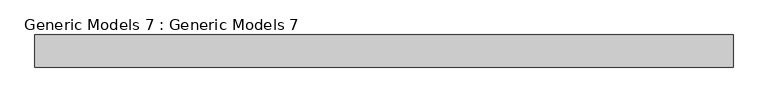
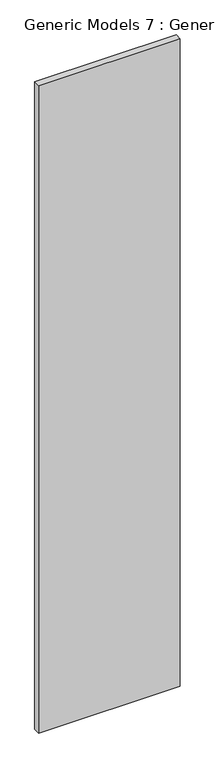
"""IFC4 building model written with IfcOpenShell, lengths in millimetres: proxy geometry, Generic Models 7 : Generic Models 7."""

from ifc_helpers import new_model, si_unit, origin, origin_with_axes, place, context, project, spatial, polyline, outline, extrude, source, transform, mapped, element, save


def generic_models_7_generic_models_7_539d4222(model_context):
    return source(origin(), model_context, "Body", "SweptSolid", [
        extrude(outline(polyline([(-6812.6326914, -4187.674389), (-8452.845593, -4187.674389), (-8452.845593, -4111.474389), (-6812.6326914, -4111.474389), (-6812.6326914, -4187.674389)])), origin_with_axes(), (0.0, 0.0, 1.0), 7924.8),
    ])


if __name__ == "__main__":
    model = new_model("IFC4")
    model_context = context("Model", 3, world=origin())
    ifc_project = project(units=[si_unit("LENGTHUNIT", "METRE", prefix="MILLI")], contexts=[model_context])
    site = spatial("IfcSite", under=ifc_project)
    building = spatial("IfcBuilding", under=site)
    placement = place(None, origin())
    generic_models_7_generic_models_7_shape = generic_models_7_generic_models_7_539d4222(model_context)
    element("IfcBuildingElementProxy", 1, Name="Generic Models 7 : Generic Models 7", ObjectType="Generic Models 7 : Generic Models 7", at=placement, inside=building, context=model_context, shape_type="MappedRepresentation", body=[
        mapped(generic_models_7_generic_models_7_shape, transform((0.0, 0.0, 0.0), x_axis=(1.0, 0.0, 0.0), y_axis=(0.0, 1.0, 0.0), z_axis=(0.0, 0.0, 1.0))),
    ])
    save(model, "model.ifc")

# Revit data of these elements
# Element 1 (IfcBuildingElementProxy, "Generic Models 7 : Generic Models 7")
#   Materials on its faces: "Asphalt Shingle"
# Materials
#   "Asphalt Shingle": class "Generic", colour RGB 155 155 155, transparency 0, Description = "Asphalt roofing shingle", Cost = 0
